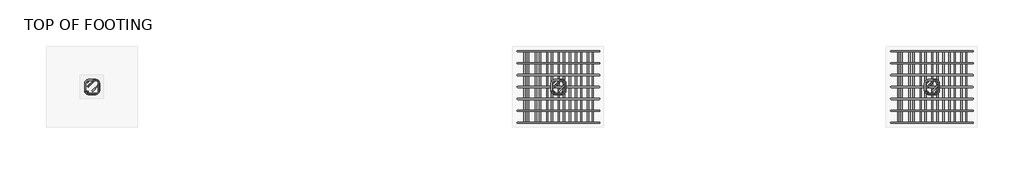
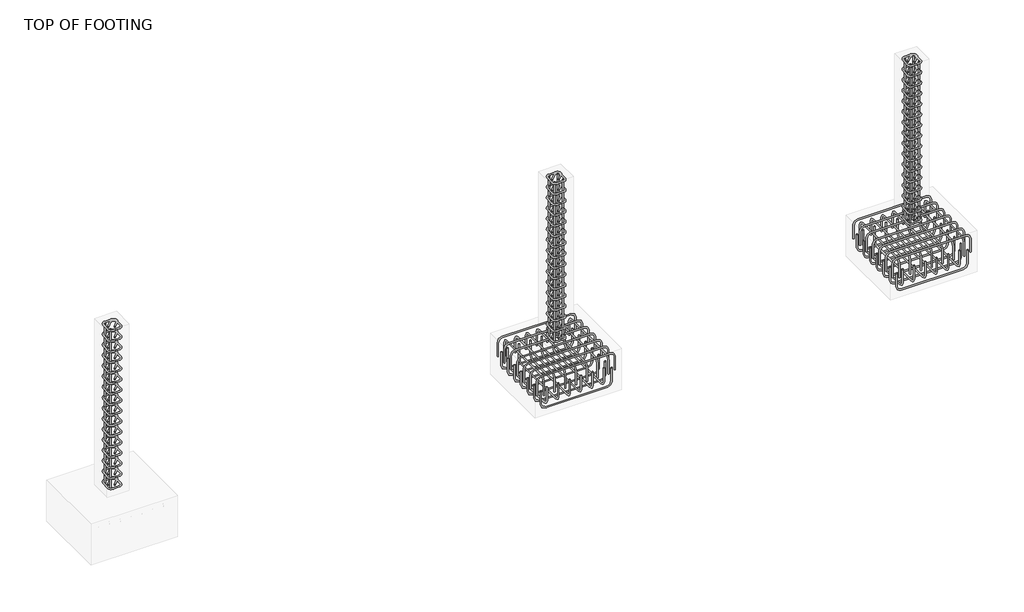
# One storey, part 6 of 6: 16 reinforcing bars.
"""IFC4 building model written with IfcOpenShell, lengths in millimetres."""

from ifc_helpers import new_model, si_unit, point, frame, origin, place, context, project, spatial, polyline, circle_curve, trimmed, segment, composite_curve, source, transform, mapped, element, save
from ifc_brep_helpers import swept_disk

model = new_model("IFC4")

# Units and contexts
model_context = context("Model", 3, world=origin())
ifc_project = project(units=[si_unit("LENGTHUNIT", "METRE", prefix="MILLI")], contexts=[model_context])

# Site, building, storey
site = spatial("IfcSite", under=ifc_project)
building = spatial("IfcBuilding", under=site)
storey = spatial("IfcBuildingStorey", under=building, Name="TOP OF FOOTING", Elevation=-1828.8)

# Reinforcing bars
placement = place(None, origin())
reinforcing_bar_shape = source(origin(), model_context, "Body", "SolidModel", [
    swept_disk(composite_curve([segment(polyline([(-6942.8971795, 4666.2516651, -2038.8), (-6942.8971795, 4666.2516651, -2186.1)]), True, "CONTINUOUS"), segment(trimmed(circle_curve(frame((-6989.2471795, 4666.2516651, -2186.1), z_axis=(0.0, 1.0, 0.0), x_axis=(46.350000000000364, 0.0, 0.0)), 46.35), [point((-6942.8971795, 4666.2516651, -2186.1))], [point((-6989.2471795, 4666.2516651, -2232.45))], True, "CARTESIAN"), True, "CONTINUOUS"), segment(polyline([(-6989.2471795, 4666.2516651, -2232.45), (-7632.3877906, 4666.2516651, -2232.45)]), True, "CONTINUOUS"), segment(trimmed(circle_curve(frame((-7632.3877906, 4666.2516651, -2186.1), z_axis=(0.0, 1.0, 0.0), x_axis=(0.0, 0.0, -46.34999999999991)), 46.35), [point((-7632.3877906, 4666.2516651, -2232.45))], [point((-7678.7377906, 4666.2516651, -2186.1))], True, "CARTESIAN"), True, "CONTINUOUS"), segment(polyline([(-7678.7377906, 4666.2516651, -2186.1), (-7678.7377906, 4666.2516651, -2038.8)]), True, "CONTINUOUS")], self_intersect=False), 6.35),
])
element("IfcReinforcingBar", 1, at=placement, inside=storey, context=model_context, shape_type="MappedRepresentation", body=[
    mapped(reinforcing_bar_shape, transform((0.0, 0.0, 0.0), x_axis=(1.0, 0.0, 0.0), y_axis=(0.0, 1.0, 0.0), z_axis=(0.0, 0.0, 1.0))),
    mapped(reinforcing_bar_shape, transform((0.0, -117.8833333, 0.0), x_axis=(1.0, 0.0, 0.0), y_axis=(0.0, 1.0, 0.0), z_axis=(0.0, 0.0, 1.0))),
    mapped(reinforcing_bar_shape, transform((0.0, -235.7666667, 0.0), x_axis=(1.0, 0.0, 0.0), y_axis=(0.0, 1.0, 0.0), z_axis=(0.0, 0.0, 1.0))),
    mapped(reinforcing_bar_shape, transform((0.0, -353.65, 0.0), x_axis=(1.0, 0.0, 0.0), y_axis=(0.0, 1.0, 0.0), z_axis=(0.0, 0.0, 1.0))),
    mapped(reinforcing_bar_shape, transform((0.0, -471.5333333, 0.0), x_axis=(1.0, 0.0, 0.0), y_axis=(0.0, 1.0, 0.0), z_axis=(0.0, 0.0, 1.0))),
    mapped(reinforcing_bar_shape, transform((0.0, -589.4166667, 0.0), x_axis=(1.0, 0.0, 0.0), y_axis=(0.0, 1.0, 0.0), z_axis=(0.0, 0.0, 1.0))),
    mapped(reinforcing_bar_shape, transform((0.0, -707.3, 0.0), x_axis=(1.0, 0.0, 0.0), y_axis=(0.0, 1.0, 0.0), z_axis=(0.0, 0.0, 1.0))),
])
reinforcing_bar_2_shape = source(origin(), model_context, "Body", "SolidModel", [
    swept_disk(composite_curve([segment(polyline([(-7718.1173382, 4666.2516651, -2070.9463075), (-7718.1173382, 4666.2516651, -1923.6463075)]), True, "CONTINUOUS"), segment(trimmed(circle_curve(frame((-7671.7673382, 4666.2516651, -1923.6463075), z_axis=(0.0, 1.0, 0.0), x_axis=(-46.349999999999454, 0.0, 0.0)), 46.35), [point((-7718.1173382, 4666.2516651, -1923.6463075))], [point((-7671.7673382, 4666.2516651, -1877.2963075))], True, "CARTESIAN"), True, "CONTINUOUS"), segment(polyline([(-7671.7673382, 4666.2516651, -1877.2963075), (-6957.1673382, 4666.2516651, -1877.2963075)]), True, "CONTINUOUS"), segment(trimmed(circle_curve(frame((-6957.1673382, 4666.2516651, -1923.6463075), z_axis=(0.0, 1.0, 0.0), x_axis=(0.0, 0.0, 46.34999999999991)), 46.35), [point((-6957.1673382, 4666.2516651, -1877.2963075))], [point((-6910.8173382, 4666.2516651, -1923.6463075))], True, "CARTESIAN"), True, "CONTINUOUS"), segment(polyline([(-6910.8173382, 4666.2516651, -1923.6463075), (-6910.8173382, 4666.2516651, -2070.9463075)]), True, "CONTINUOUS")], self_intersect=False), 6.35),
])
element("IfcReinforcingBar", 2, at=placement, inside=storey, context=model_context, shape_type="MappedRepresentation", body=[
    mapped(reinforcing_bar_2_shape, transform((0.0, 0.0, 0.0), x_axis=(1.0, 0.0, 0.0), y_axis=(0.0, 1.0, 0.0), z_axis=(0.0, 0.0, 1.0))),
    mapped(reinforcing_bar_2_shape, transform((0.0, -117.8833333, 0.0), x_axis=(1.0, 0.0, 0.0), y_axis=(0.0, 1.0, 0.0), z_axis=(0.0, 0.0, 1.0))),
    mapped(reinforcing_bar_2_shape, transform((0.0, -235.7666667, 0.0), x_axis=(1.0, 0.0, 0.0), y_axis=(0.0, 1.0, 0.0), z_axis=(0.0, 0.0, 1.0))),
    mapped(reinforcing_bar_2_shape, transform((0.0, -353.65, 0.0), x_axis=(1.0, 0.0, 0.0), y_axis=(0.0, 1.0, 0.0), z_axis=(0.0, 0.0, 1.0))),
    mapped(reinforcing_bar_2_shape, transform((0.0, -471.5333333, 0.0), x_axis=(1.0, 0.0, 0.0), y_axis=(0.0, 1.0, 0.0), z_axis=(0.0, 0.0, 1.0))),
    mapped(reinforcing_bar_2_shape, transform((0.0, -589.4166667, 0.0), x_axis=(1.0, 0.0, 0.0), y_axis=(0.0, 1.0, 0.0), z_axis=(0.0, 0.0, 1.0))),
    mapped(reinforcing_bar_2_shape, transform((0.0, -707.3, 0.0), x_axis=(1.0, 0.0, 0.0), y_axis=(0.0, 1.0, 0.0), z_axis=(0.0, 0.0, 1.0))),
])
reinforcing_bar_3_shape = source(origin(), model_context, "Body", "SolidModel", [
    swept_disk(composite_curve([segment(polyline([(-6975.9662545, 4666.2516651, -2094.0228735), (-6975.9662545, 4666.2516651, -1946.7228735)]), True, "CONTINUOUS"), segment(trimmed(circle_curve(frame((-6975.9662545, 4619.9016651, -1946.7228735), z_axis=(1.0, 0.0, 0.0), x_axis=(0.0, 46.349999999999454, 0.0)), 46.35), [point((-6975.9662545, 4666.2516651, -1946.7228735))], [point((-6975.9662545, 4619.9016651, -1900.3728735))], True, "CARTESIAN"), True, "CONTINUOUS"), segment(polyline([(-6975.9662545, 4619.9016651, -1900.3728735), (-6975.9662545, 4005.3016651, -1900.3728735)]), True, "CONTINUOUS"), segment(trimmed(circle_curve(frame((-6975.9662545, 4005.3016651, -1946.7228735), z_axis=(1.0, 0.0, 0.0), x_axis=(0.0, 0.0, 46.350000000000136)), 46.35), [point((-6975.9662545, 4005.3016651, -1900.3728735))], [point((-6975.9662545, 3958.9516651, -1946.7228735))], True, "CARTESIAN"), True, "CONTINUOUS"), segment(polyline([(-6975.9662545, 3958.9516651, -1946.7228735), (-6975.9662545, 3958.9516651, -2094.0228735)]), True, "CONTINUOUS")], self_intersect=False), 6.35),
])
element("IfcReinforcingBar", 3, at=placement, inside=storey, context=model_context, shape_type="MappedRepresentation", body=[
    mapped(reinforcing_bar_3_shape, transform((0.0, 0.0, 0.0), x_axis=(1.0, 0.0, 0.0), y_axis=(0.0, 1.0, 0.0), z_axis=(0.0, 0.0, 1.0))),
    mapped(reinforcing_bar_3_shape, transform((-112.124631, 0.0, 0.0), x_axis=(1.0, 0.0, 0.0), y_axis=(0.0, 1.0, 0.0), z_axis=(0.0, 0.0, 1.0))),
    mapped(reinforcing_bar_3_shape, transform((-224.2492621, 0.0, 0.0), x_axis=(1.0, 0.0, 0.0), y_axis=(0.0, 1.0, 0.0), z_axis=(0.0, 0.0, 1.0))),
    mapped(reinforcing_bar_3_shape, transform((-336.3738931, 0.0, 0.0), x_axis=(1.0, 0.0, 0.0), y_axis=(0.0, 1.0, 0.0), z_axis=(0.0, 0.0, 1.0))),
    mapped(reinforcing_bar_3_shape, transform((-448.4985241, 0.0, 0.0), x_axis=(1.0, 0.0, 0.0), y_axis=(0.0, 1.0, 0.0), z_axis=(0.0, 0.0, 1.0))),
    mapped(reinforcing_bar_3_shape, transform((-560.6231552, 0.0, 0.0), x_axis=(1.0, 0.0, 0.0), y_axis=(0.0, 1.0, 0.0), z_axis=(0.0, 0.0, 1.0))),
    mapped(reinforcing_bar_3_shape, transform((-672.7477862, 0.0, 0.0), x_axis=(1.0, 0.0, 0.0), y_axis=(0.0, 1.0, 0.0), z_axis=(0.0, 0.0, 1.0))),
])
reinforcing_bar_4_shape = source(origin(), model_context, "Body", "SolidModel", [
    swept_disk(composite_curve([segment(polyline([(-7615.9564967, 4666.2516651, -2014.7438142), (-7615.9564967, 4666.2516651, -2162.0438142)]), True, "CONTINUOUS"), segment(trimmed(circle_curve(frame((-7615.9564967, 4619.9016651, -2162.0438142), z_axis=(-1.0, 0.0, 0.0), x_axis=(0.0, 46.349999999999454, 0.0)), 46.35), [point((-7615.9564967, 4666.2516651, -2162.0438142))], [point((-7615.9564967, 4619.9016651, -2208.3938142))], True, "CARTESIAN"), True, "CONTINUOUS"), segment(polyline([(-7615.9564967, 4619.9016651, -2208.3938142), (-7615.9564967, 4005.3016651, -2208.3938142)]), True, "CONTINUOUS"), segment(trimmed(circle_curve(frame((-7615.9564967, 4005.3016651, -2162.0438142), z_axis=(-1.0, 0.0, 0.0), x_axis=(0.0, 0.0, -46.350000000000364)), 46.35), [point((-7615.9564967, 4005.3016651, -2208.3938142))], [point((-7615.9564967, 3958.9516651, -2162.0438142))], True, "CARTESIAN"), True, "CONTINUOUS"), segment(polyline([(-7615.9564967, 3958.9516651, -2162.0438142), (-7615.9564967, 3958.9516651, -2014.7438142)]), True, "CONTINUOUS")], self_intersect=False), 6.35),
])
element("IfcReinforcingBar", 4, at=placement, inside=storey, context=model_context, shape_type="MappedRepresentation", body=[
    mapped(reinforcing_bar_4_shape, transform((0.0, 0.0, 0.0), x_axis=(1.0, 0.0, 0.0), y_axis=(0.0, 1.0, 0.0), z_axis=(0.0, 0.0, 1.0))),
    mapped(reinforcing_bar_4_shape, transform((118.647936, 0.0, 0.0), x_axis=(1.0, 0.0, 0.0), y_axis=(0.0, 1.0, 0.0), z_axis=(0.0, 0.0, 1.0))),
    mapped(reinforcing_bar_4_shape, transform((237.295872, 0.0, 0.0), x_axis=(1.0, 0.0, 0.0), y_axis=(0.0, 1.0, 0.0), z_axis=(0.0, 0.0, 1.0))),
    mapped(reinforcing_bar_4_shape, transform((355.943808, 0.0, 0.0), x_axis=(1.0, 0.0, 0.0), y_axis=(0.0, 1.0, 0.0), z_axis=(0.0, 0.0, 1.0))),
    mapped(reinforcing_bar_4_shape, transform((474.591744, 0.0, 0.0), x_axis=(1.0, 0.0, 0.0), y_axis=(0.0, 1.0, 0.0), z_axis=(0.0, 0.0, 1.0))),
    mapped(reinforcing_bar_4_shape, transform((593.23968, 0.0, 0.0), x_axis=(1.0, 0.0, 0.0), y_axis=(0.0, 1.0, 0.0), z_axis=(0.0, 0.0, 1.0))),
])
reinforcing_bar_5_shape = source(origin(), model_context, "Body", "SolidModel", [
    swept_disk(composite_curve([segment(polyline([(-3249.1855212, 4666.2516651, -2038.8), (-3249.1855212, 4666.2516651, -2186.1)]), True, "CONTINUOUS"), segment(trimmed(circle_curve(frame((-3295.5355212, 4666.2516651, -2186.1), z_axis=(0.0, 1.0, 0.0), x_axis=(46.34999999999991, 0.0, 0.0)), 46.35), [point((-3249.1855212, 4666.2516651, -2186.1))], [point((-3295.5355212, 4666.2516651, -2232.45))], True, "CARTESIAN"), True, "CONTINUOUS"), segment(polyline([(-3295.5355212, 4666.2516651, -2232.45), (-3938.6761323, 4666.2516651, -2232.45)]), True, "CONTINUOUS"), segment(trimmed(circle_curve(frame((-3938.6761323, 4666.2516651, -2186.1), z_axis=(0.0, 1.0, 0.0), x_axis=(0.0, 0.0, -46.34999999999991)), 46.35), [point((-3938.6761323, 4666.2516651, -2232.45))], [point((-3985.0261323, 4666.2516651, -2186.1))], True, "CARTESIAN"), True, "CONTINUOUS"), segment(polyline([(-3985.0261323, 4666.2516651, -2186.1), (-3985.0261323, 4666.2516651, -2038.8)]), True, "CONTINUOUS")], self_intersect=False), 6.35),
])
element("IfcReinforcingBar", 5, at=placement, inside=storey, context=model_context, shape_type="MappedRepresentation", body=[
    mapped(reinforcing_bar_5_shape, transform((0.0, 0.0, 0.0), x_axis=(1.0, 0.0, 0.0), y_axis=(0.0, 1.0, 0.0), z_axis=(0.0, 0.0, 1.0))),
    mapped(reinforcing_bar_5_shape, transform((0.0, -117.8833333, 0.0), x_axis=(1.0, 0.0, 0.0), y_axis=(0.0, 1.0, 0.0), z_axis=(0.0, 0.0, 1.0))),
    mapped(reinforcing_bar_5_shape, transform((0.0, -235.7666667, 0.0), x_axis=(1.0, 0.0, 0.0), y_axis=(0.0, 1.0, 0.0), z_axis=(0.0, 0.0, 1.0))),
    mapped(reinforcing_bar_5_shape, transform((0.0, -353.65, 0.0), x_axis=(1.0, 0.0, 0.0), y_axis=(0.0, 1.0, 0.0), z_axis=(0.0, 0.0, 1.0))),
    mapped(reinforcing_bar_5_shape, transform((0.0, -471.5333333, 0.0), x_axis=(1.0, 0.0, 0.0), y_axis=(0.0, 1.0, 0.0), z_axis=(0.0, 0.0, 1.0))),
    mapped(reinforcing_bar_5_shape, transform((0.0, -589.4166667, 0.0), x_axis=(1.0, 0.0, 0.0), y_axis=(0.0, 1.0, 0.0), z_axis=(0.0, 0.0, 1.0))),
    mapped(reinforcing_bar_5_shape, transform((0.0, -707.3, 0.0), x_axis=(1.0, 0.0, 0.0), y_axis=(0.0, 1.0, 0.0), z_axis=(0.0, 0.0, 1.0))),
])
reinforcing_bar_6_shape = source(origin(), model_context, "Body", "SolidModel", [
    swept_disk(composite_curve([segment(polyline([(-4024.4056799, 4666.2516651, -2070.9463075), (-4024.4056799, 4666.2516651, -1923.6463075)]), True, "CONTINUOUS"), segment(trimmed(circle_curve(frame((-3978.0556799, 4666.2516651, -1923.6463075), z_axis=(0.0, 1.0, 0.0), x_axis=(-46.34999999999991, 0.0, 0.0)), 46.35), [point((-4024.4056799, 4666.2516651, -1923.6463075))], [point((-3978.0556799, 4666.2516651, -1877.2963075))], True, "CARTESIAN"), True, "CONTINUOUS"), segment(polyline([(-3978.0556799, 4666.2516651, -1877.2963075), (-3263.4556799, 4666.2516651, -1877.2963075)]), True, "CONTINUOUS"), segment(trimmed(circle_curve(frame((-3263.4556799, 4666.2516651, -1923.6463075), z_axis=(0.0, 1.0, 0.0), x_axis=(0.0, 0.0, 46.34999999999991)), 46.35), [point((-3263.4556799, 4666.2516651, -1877.2963075))], [point((-3217.1056799, 4666.2516651, -1923.6463075))], True, "CARTESIAN"), True, "CONTINUOUS"), segment(polyline([(-3217.1056799, 4666.2516651, -1923.6463075), (-3217.1056799, 4666.2516651, -2070.9463075)]), True, "CONTINUOUS")], self_intersect=False), 6.35),
])
element("IfcReinforcingBar", 6, at=placement, inside=storey, context=model_context, shape_type="MappedRepresentation", body=[
    mapped(reinforcing_bar_6_shape, transform((0.0, 0.0, 0.0), x_axis=(1.0, 0.0, 0.0), y_axis=(0.0, 1.0, 0.0), z_axis=(0.0, 0.0, 1.0))),
    mapped(reinforcing_bar_6_shape, transform((0.0, -117.8833333, 0.0), x_axis=(1.0, 0.0, 0.0), y_axis=(0.0, 1.0, 0.0), z_axis=(0.0, 0.0, 1.0))),
    mapped(reinforcing_bar_6_shape, transform((0.0, -235.7666667, 0.0), x_axis=(1.0, 0.0, 0.0), y_axis=(0.0, 1.0, 0.0), z_axis=(0.0, 0.0, 1.0))),
    mapped(reinforcing_bar_6_shape, transform((0.0, -353.65, 0.0), x_axis=(1.0, 0.0, 0.0), y_axis=(0.0, 1.0, 0.0), z_axis=(0.0, 0.0, 1.0))),
    mapped(reinforcing_bar_6_shape, transform((0.0, -471.5333333, 0.0), x_axis=(1.0, 0.0, 0.0), y_axis=(0.0, 1.0, 0.0), z_axis=(0.0, 0.0, 1.0))),
    mapped(reinforcing_bar_6_shape, transform((0.0, -589.4166667, 0.0), x_axis=(1.0, 0.0, 0.0), y_axis=(0.0, 1.0, 0.0), z_axis=(0.0, 0.0, 1.0))),
    mapped(reinforcing_bar_6_shape, transform((0.0, -707.3, 0.0), x_axis=(1.0, 0.0, 0.0), y_axis=(0.0, 1.0, 0.0), z_axis=(0.0, 0.0, 1.0))),
])
reinforcing_bar_7_shape = source(origin(), model_context, "Body", "SolidModel", [
    swept_disk(composite_curve([segment(polyline([(-3282.2545962, 4666.2516651, -2094.0228735), (-3282.2545962, 4666.2516651, -1946.7228735)]), True, "CONTINUOUS"), segment(trimmed(circle_curve(frame((-3282.2545962, 4619.9016651, -1946.7228735), z_axis=(1.0, 0.0, 0.0), x_axis=(0.0, 46.349999999999454, 0.0)), 46.35), [point((-3282.2545962, 4666.2516651, -1946.7228735))], [point((-3282.2545962, 4619.9016651, -1900.3728735))], True, "CARTESIAN"), True, "CONTINUOUS"), segment(polyline([(-3282.2545962, 4619.9016651, -1900.3728735), (-3282.2545962, 4005.3016651, -1900.3728735)]), True, "CONTINUOUS"), segment(trimmed(circle_curve(frame((-3282.2545962, 4005.3016651, -1946.7228735), z_axis=(1.0, 0.0, 0.0), x_axis=(0.0, 0.0, 46.350000000000136)), 46.35), [point((-3282.2545962, 4005.3016651, -1900.3728735))], [point((-3282.2545962, 3958.9516651, -1946.7228735))], True, "CARTESIAN"), True, "CONTINUOUS"), segment(polyline([(-3282.2545962, 3958.9516651, -1946.7228735), (-3282.2545962, 3958.9516651, -2094.0228735)]), True, "CONTINUOUS")], self_intersect=False), 6.35),
])
element("IfcReinforcingBar", 7, at=placement, inside=storey, context=model_context, shape_type="MappedRepresentation", body=[
    mapped(reinforcing_bar_7_shape, transform((0.0, 0.0, 0.0), x_axis=(1.0, 0.0, 0.0), y_axis=(0.0, 1.0, 0.0), z_axis=(0.0, 0.0, 1.0))),
    mapped(reinforcing_bar_7_shape, transform((-112.124631, 0.0, 0.0), x_axis=(1.0, 0.0, 0.0), y_axis=(0.0, 1.0, 0.0), z_axis=(0.0, 0.0, 1.0))),
    mapped(reinforcing_bar_7_shape, transform((-224.2492621, 0.0, 0.0), x_axis=(1.0, 0.0, 0.0), y_axis=(0.0, 1.0, 0.0), z_axis=(0.0, 0.0, 1.0))),
    mapped(reinforcing_bar_7_shape, transform((-336.3738931, 0.0, 0.0), x_axis=(1.0, 0.0, 0.0), y_axis=(0.0, 1.0, 0.0), z_axis=(0.0, 0.0, 1.0))),
    mapped(reinforcing_bar_7_shape, transform((-448.4985241, 0.0, 0.0), x_axis=(1.0, 0.0, 0.0), y_axis=(0.0, 1.0, 0.0), z_axis=(0.0, 0.0, 1.0))),
    mapped(reinforcing_bar_7_shape, transform((-560.6231552, 0.0, 0.0), x_axis=(1.0, 0.0, 0.0), y_axis=(0.0, 1.0, 0.0), z_axis=(0.0, 0.0, 1.0))),
    mapped(reinforcing_bar_7_shape, transform((-672.7477862, 0.0, 0.0), x_axis=(1.0, 0.0, 0.0), y_axis=(0.0, 1.0, 0.0), z_axis=(0.0, 0.0, 1.0))),
])
reinforcing_bar_8_shape = source(origin(), model_context, "Body", "SolidModel", [
    swept_disk(composite_curve([segment(polyline([(-3922.2448384, 4666.2516651, -2014.7438142), (-3922.2448384, 4666.2516651, -2162.0438142)]), True, "CONTINUOUS"), segment(trimmed(circle_curve(frame((-3922.2448384, 4619.9016651, -2162.0438142), z_axis=(-1.0, 0.0, 0.0), x_axis=(0.0, 46.349999999999454, 0.0)), 46.35), [point((-3922.2448384, 4666.2516651, -2162.0438142))], [point((-3922.2448384, 4619.9016651, -2208.3938142))], True, "CARTESIAN"), True, "CONTINUOUS"), segment(polyline([(-3922.2448384, 4619.9016651, -2208.3938142), (-3922.2448384, 4005.3016651, -2208.3938142)]), True, "CONTINUOUS"), segment(trimmed(circle_curve(frame((-3922.2448384, 4005.3016651, -2162.0438142), z_axis=(-1.0, 0.0, 0.0), x_axis=(0.0, 0.0, -46.350000000000364)), 46.35), [point((-3922.2448384, 4005.3016651, -2208.3938142))], [point((-3922.2448384, 3958.9516651, -2162.0438142))], True, "CARTESIAN"), True, "CONTINUOUS"), segment(polyline([(-3922.2448384, 3958.9516651, -2162.0438142), (-3922.2448384, 3958.9516651, -2014.7438142)]), True, "CONTINUOUS")], self_intersect=False), 6.35),
])
element("IfcReinforcingBar", 8, at=placement, inside=storey, context=model_context, shape_type="MappedRepresentation", body=[
    mapped(reinforcing_bar_8_shape, transform((0.0, 0.0, 0.0), x_axis=(1.0, 0.0, 0.0), y_axis=(0.0, 1.0, 0.0), z_axis=(0.0, 0.0, 1.0))),
    mapped(reinforcing_bar_8_shape, transform((118.647936, 0.0, 0.0), x_axis=(1.0, 0.0, 0.0), y_axis=(0.0, 1.0, 0.0), z_axis=(0.0, 0.0, 1.0))),
    mapped(reinforcing_bar_8_shape, transform((237.295872, 0.0, 0.0), x_axis=(1.0, 0.0, 0.0), y_axis=(0.0, 1.0, 0.0), z_axis=(0.0, 0.0, 1.0))),
    mapped(reinforcing_bar_8_shape, transform((355.943808, 0.0, 0.0), x_axis=(1.0, 0.0, 0.0), y_axis=(0.0, 1.0, 0.0), z_axis=(0.0, 0.0, 1.0))),
    mapped(reinforcing_bar_8_shape, transform((474.591744, 0.0, 0.0), x_axis=(1.0, 0.0, 0.0), y_axis=(0.0, 1.0, 0.0), z_axis=(0.0, 0.0, 1.0))),
    mapped(reinforcing_bar_8_shape, transform((593.23968, 0.0, 0.0), x_axis=(1.0, 0.0, 0.0), y_axis=(0.0, 1.0, 0.0), z_axis=(0.0, 0.0, 1.0))),
])
reinforcing_bar_9_shape = source(origin(), model_context, "Body", "SolidModel", [
    swept_disk(composite_curve([segment(polyline([(-3576.0006936, 4361.3993608, -40.0), (-3576.0006936, 4361.3993608, -1788.8)]), True, "CONTINUOUS")], self_intersect=False), 6.35),
])
element("IfcReinforcingBar", 9, at=placement, inside=storey, context=model_context, shape_type="MappedRepresentation", body=[
    mapped(reinforcing_bar_9_shape, transform((0.0, 0.0, 0.0), x_axis=(1.0, 0.0, 0.0), y_axis=(0.0, 1.0, 0.0), z_axis=(0.0, 0.0, 1.0))),
    mapped(reinforcing_bar_9_shape, transform((0.0, -96.9916148, 0.0), x_axis=(1.0, 0.0, 0.0), y_axis=(0.0, 1.0, 0.0), z_axis=(0.0, 0.0, 1.0))),
])
reinforcing_bar_10_shape = source(origin(), model_context, "Body", "SolidModel", [
    swept_disk(composite_curve([segment(polyline([(-3662.0670404, 4315.6258997, -46.35), (-3606.3234775, 4371.3694627, -46.35)]), True, "CONTINUOUS"), segment(trimmed(circle_curve(frame((-3584.1556799, 4349.2016651, -46.35), z_axis=(0.0, 0.0, -1.0), x_axis=(-22.167797600000085, 22.167797600000085, 0.0)), 31.35), [point((-3606.3234775, 4371.3694627, -46.35))], [point((-3552.8056799, 4349.2016651, -46.35))], True, "CARTESIAN"), True, "CONTINUOUS"), segment(polyline([(-3552.8056799, 4349.2016651, -46.35), (-3552.8056799, 4276.0016651, -46.35)]), True, "CONTINUOUS"), segment(trimmed(circle_curve(frame((-3584.1556799, 4276.0016651, -46.35), z_axis=(0.0, 0.0, -1.0), x_axis=(31.34999999999991, 0.0, 0.0)), 31.35), [point((-3552.8056799, 4276.0016651, -46.35))], [point((-3584.1556799, 4244.6516651, -46.35))], True, "CARTESIAN"), True, "CONTINUOUS"), segment(polyline([(-3584.1556799, 4244.6516651, -46.35), (-3657.3556799, 4244.6516651, -46.35)]), True, "CONTINUOUS"), segment(trimmed(circle_curve(frame((-3657.3556799, 4275.8656639, -43.4330185), z_axis=(0.0, 0.09304566152621355, -0.9956618426308951), x_axis=(0.0, -31.2139987999999, -2.9169814999999986)), 31.35), [point((-3657.3556799, 4244.6516651, -46.35))], [point((-3688.7056799, 4275.8656639, -43.4330185))], True, "CARTESIAN"), True, "CONTINUOUS"), segment(polyline([(-3688.7056799, 4275.8656639, -43.4330185), (-3688.7056799, 4349.3376663, -36.5669815)]), True, "CONTINUOUS"), segment(trimmed(circle_curve(frame((-3657.3556799, 4349.3376663, -36.5669815), z_axis=(0.0, 0.09304566152621355, -0.9956618426308951), x_axis=(-31.350000000000364, 0.0, 0.0)), 31.35), [point((-3688.7056799, 4349.3376663, -36.5669815))], [point((-3657.3556799, 4380.5516651, -33.65))], True, "CARTESIAN"), True, "CONTINUOUS"), segment(polyline([(-3657.3556799, 4380.5516651, -33.65), (-3584.1556799, 4380.5516651, -33.65)]), True, "CONTINUOUS"), segment(trimmed(circle_curve(frame((-3584.1556799, 4349.2016651, -33.65), z_axis=(0.0, 0.0, -1.0), x_axis=(0.0, 31.349999999999454, 0.0)), 31.35), [point((-3584.1556799, 4380.5516651, -33.65))], [point((-3561.9878823, 4327.0338675, -33.65))], True, "CARTESIAN"), True, "CONTINUOUS"), segment(polyline([(-3561.9878823, 4327.0338675, -33.65), (-3617.7314452, 4271.2903046, -33.65)]), True, "CONTINUOUS")], self_intersect=False), 6.35),
])
element("IfcReinforcingBar", 10, at=placement, inside=storey, context=model_context, shape_type="MappedRepresentation", body=[
    mapped(reinforcing_bar_10_shape, transform((0.0, 0.0, 0.0), x_axis=(1.0, 0.0, 0.0), y_axis=(0.0, 1.0, 0.0), z_axis=(0.0, 0.0, 1.0))),
    mapped(reinforcing_bar_10_shape, transform((0.0, 0.0, -115.74), x_axis=(1.0, 0.0, 0.0), y_axis=(0.0, 1.0, 0.0), z_axis=(0.0, 0.0, 1.0))),
    mapped(reinforcing_bar_10_shape, transform((0.0, 0.0, -231.48), x_axis=(1.0, 0.0, 0.0), y_axis=(0.0, 1.0, 0.0), z_axis=(0.0, 0.0, 1.0))),
    mapped(reinforcing_bar_10_shape, transform((0.0, 0.0, -347.22), x_axis=(1.0, 0.0, 0.0), y_axis=(0.0, 1.0, 0.0), z_axis=(0.0, 0.0, 1.0))),
    mapped(reinforcing_bar_10_shape, transform((0.0, 0.0, -462.96), x_axis=(1.0, 0.0, 0.0), y_axis=(0.0, 1.0, 0.0), z_axis=(0.0, 0.0, 1.0))),
    mapped(reinforcing_bar_10_shape, transform((0.0, 0.0, -578.7), x_axis=(1.0, 0.0, 0.0), y_axis=(0.0, 1.0, 0.0), z_axis=(0.0, 0.0, 1.0))),
    mapped(reinforcing_bar_10_shape, transform((0.0, 0.0, -694.44), x_axis=(1.0, 0.0, 0.0), y_axis=(0.0, 1.0, 0.0), z_axis=(0.0, 0.0, 1.0))),
    mapped(reinforcing_bar_10_shape, transform((0.0, 0.0, -810.18), x_axis=(1.0, 0.0, 0.0), y_axis=(0.0, 1.0, 0.0), z_axis=(0.0, 0.0, 1.0))),
    mapped(reinforcing_bar_10_shape, transform((0.0, 0.0, -925.92), x_axis=(1.0, 0.0, 0.0), y_axis=(0.0, 1.0, 0.0), z_axis=(0.0, 0.0, 1.0))),
    mapped(reinforcing_bar_10_shape, transform((0.0, 0.0, -1041.66), x_axis=(1.0, 0.0, 0.0), y_axis=(0.0, 1.0, 0.0), z_axis=(0.0, 0.0, 1.0))),
    mapped(reinforcing_bar_10_shape, transform((0.0, 0.0, -1157.4), x_axis=(1.0, 0.0, 0.0), y_axis=(0.0, 1.0, 0.0), z_axis=(0.0, 0.0, 1.0))),
    mapped(reinforcing_bar_10_shape, transform((0.0, 0.0, -1273.14), x_axis=(1.0, 0.0, 0.0), y_axis=(0.0, 1.0, 0.0), z_axis=(0.0, 0.0, 1.0))),
    mapped(reinforcing_bar_10_shape, transform((0.0, 0.0, -1388.88), x_axis=(1.0, 0.0, 0.0), y_axis=(0.0, 1.0, 0.0), z_axis=(0.0, 0.0, 1.0))),
    mapped(reinforcing_bar_10_shape, transform((0.0, 0.0, -1504.62), x_axis=(1.0, 0.0, 0.0), y_axis=(0.0, 1.0, 0.0), z_axis=(0.0, 0.0, 1.0))),
    mapped(reinforcing_bar_10_shape, transform((0.0, 0.0, -1620.36), x_axis=(1.0, 0.0, 0.0), y_axis=(0.0, 1.0, 0.0), z_axis=(0.0, 0.0, 1.0))),
    mapped(reinforcing_bar_10_shape, transform((0.0, 0.0, -1736.1), x_axis=(1.0, 0.0, 0.0), y_axis=(0.0, 1.0, 0.0), z_axis=(0.0, 0.0, 1.0))),
])
reinforcing_bar_11_shape = source(origin(), model_context, "Body", "SolidModel", [
    swept_disk(composite_curve([segment(polyline([(-3665.5106662, 4361.3993608, -40.0), (-3665.5106662, 4361.3993608, -1788.8)]), True, "CONTINUOUS")], self_intersect=False), 6.35),
])
element("IfcReinforcingBar", 11, at=placement, inside=storey, context=model_context, shape_type="MappedRepresentation", body=[
    mapped(reinforcing_bar_11_shape, transform((0.0, 0.0, 0.0), x_axis=(1.0, 0.0, 0.0), y_axis=(0.0, 1.0, 0.0), z_axis=(0.0, 0.0, 1.0))),
    mapped(reinforcing_bar_11_shape, transform((0.0, -96.9916148, 0.0), x_axis=(1.0, 0.0, 0.0), y_axis=(0.0, 1.0, 0.0), z_axis=(0.0, 0.0, 1.0))),
])
reinforcing_bar_12_shape = source(origin(), model_context, "Body", "SolidModel", [
    swept_disk(composite_curve([segment(polyline([(-7269.7123519, 4361.3993608, -40.0), (-7269.7123519, 4361.3993608, -1788.8)]), True, "CONTINUOUS")], self_intersect=False), 6.35),
])
element("IfcReinforcingBar", 12, at=placement, inside=storey, context=model_context, shape_type="MappedRepresentation", body=[
    mapped(reinforcing_bar_12_shape, transform((0.0, 0.0, 0.0), x_axis=(1.0, 0.0, 0.0), y_axis=(0.0, 1.0, 0.0), z_axis=(0.0, 0.0, 1.0))),
    mapped(reinforcing_bar_12_shape, transform((0.0, -96.9916148, 0.0), x_axis=(1.0, 0.0, 0.0), y_axis=(0.0, 1.0, 0.0), z_axis=(0.0, 0.0, 1.0))),
])
reinforcing_bar_13_shape = source(origin(), model_context, "Body", "SolidModel", [
    swept_disk(composite_curve([segment(polyline([(-7355.7786987, 4315.6258997, -46.35), (-7300.0351358, 4371.3694627, -46.35)]), True, "CONTINUOUS"), segment(trimmed(circle_curve(frame((-7277.8673382, 4349.2016651, -46.35), z_axis=(0.0, 0.0, -1.0), x_axis=(-22.167797600000085, 22.167797600000085, 0.0)), 31.35), [point((-7300.0351358, 4371.3694627, -46.35))], [point((-7246.5173382, 4349.2016651, -46.35))], True, "CARTESIAN"), True, "CONTINUOUS"), segment(polyline([(-7246.5173382, 4349.2016651, -46.35), (-7246.5173382, 4276.0016651, -46.35)]), True, "CONTINUOUS"), segment(trimmed(circle_curve(frame((-7277.8673382, 4276.0016651, -46.35), z_axis=(0.0, 0.0, -1.0), x_axis=(31.349999999999454, 0.0, 0.0)), 31.35), [point((-7246.5173382, 4276.0016651, -46.35))], [point((-7277.8673382, 4244.6516651, -46.35))], True, "CARTESIAN"), True, "CONTINUOUS"), segment(polyline([(-7277.8673382, 4244.6516651, -46.35), (-7351.0673382, 4244.6516651, -46.35)]), True, "CONTINUOUS"), segment(trimmed(circle_curve(frame((-7351.0673382, 4275.8656639, -43.4330185), z_axis=(0.0, 0.09304566152621355, -0.9956618426308951), x_axis=(0.0, -31.2139987999999, -2.9169814999999986)), 31.35), [point((-7351.0673382, 4244.6516651, -46.35))], [point((-7382.4173382, 4275.8656639, -43.4330185))], True, "CARTESIAN"), True, "CONTINUOUS"), segment(polyline([(-7382.4173382, 4275.8656639, -43.4330185), (-7382.4173382, 4349.3376663, -36.5669815)]), True, "CONTINUOUS"), segment(trimmed(circle_curve(frame((-7351.0673382, 4349.3376663, -36.5669815), z_axis=(0.0, 0.09304566152621355, -0.9956618426308951), x_axis=(-31.349999999999454, 0.0, 0.0)), 31.35), [point((-7382.4173382, 4349.3376663, -36.5669815))], [point((-7351.0673382, 4380.5516651, -33.65))], True, "CARTESIAN"), True, "CONTINUOUS"), segment(polyline([(-7351.0673382, 4380.5516651, -33.65), (-7277.8673382, 4380.5516651, -33.65)]), True, "CONTINUOUS"), segment(trimmed(circle_curve(frame((-7277.8673382, 4349.2016651, -33.65), z_axis=(0.0, 0.0, -1.0), x_axis=(0.0, 31.349999999999454, 0.0)), 31.35), [point((-7277.8673382, 4380.5516651, -33.65))], [point((-7255.6995406, 4327.0338675, -33.65))], True, "CARTESIAN"), True, "CONTINUOUS"), segment(polyline([(-7255.6995406, 4327.0338675, -33.65), (-7311.4431035, 4271.2903046, -33.65)]), True, "CONTINUOUS")], self_intersect=False), 6.35),
])
element("IfcReinforcingBar", 13, at=placement, inside=storey, context=model_context, shape_type="MappedRepresentation", body=[
    mapped(reinforcing_bar_13_shape, transform((0.0, 0.0, 0.0), x_axis=(1.0, 0.0, 0.0), y_axis=(0.0, 1.0, 0.0), z_axis=(0.0, 0.0, 1.0))),
    mapped(reinforcing_bar_13_shape, transform((0.0, 0.0, -115.74), x_axis=(1.0, 0.0, 0.0), y_axis=(0.0, 1.0, 0.0), z_axis=(0.0, 0.0, 1.0))),
    mapped(reinforcing_bar_13_shape, transform((0.0, 0.0, -231.48), x_axis=(1.0, 0.0, 0.0), y_axis=(0.0, 1.0, 0.0), z_axis=(0.0, 0.0, 1.0))),
    mapped(reinforcing_bar_13_shape, transform((0.0, 0.0, -347.22), x_axis=(1.0, 0.0, 0.0), y_axis=(0.0, 1.0, 0.0), z_axis=(0.0, 0.0, 1.0))),
    mapped(reinforcing_bar_13_shape, transform((0.0, 0.0, -462.96), x_axis=(1.0, 0.0, 0.0), y_axis=(0.0, 1.0, 0.0), z_axis=(0.0, 0.0, 1.0))),
    mapped(reinforcing_bar_13_shape, transform((0.0, 0.0, -578.7), x_axis=(1.0, 0.0, 0.0), y_axis=(0.0, 1.0, 0.0), z_axis=(0.0, 0.0, 1.0))),
    mapped(reinforcing_bar_13_shape, transform((0.0, 0.0, -694.44), x_axis=(1.0, 0.0, 0.0), y_axis=(0.0, 1.0, 0.0), z_axis=(0.0, 0.0, 1.0))),
    mapped(reinforcing_bar_13_shape, transform((0.0, 0.0, -810.18), x_axis=(1.0, 0.0, 0.0), y_axis=(0.0, 1.0, 0.0), z_axis=(0.0, 0.0, 1.0))),
    mapped(reinforcing_bar_13_shape, transform((0.0, 0.0, -925.92), x_axis=(1.0, 0.0, 0.0), y_axis=(0.0, 1.0, 0.0), z_axis=(0.0, 0.0, 1.0))),
    mapped(reinforcing_bar_13_shape, transform((0.0, 0.0, -1041.66), x_axis=(1.0, 0.0, 0.0), y_axis=(0.0, 1.0, 0.0), z_axis=(0.0, 0.0, 1.0))),
    mapped(reinforcing_bar_13_shape, transform((0.0, 0.0, -1157.4), x_axis=(1.0, 0.0, 0.0), y_axis=(0.0, 1.0, 0.0), z_axis=(0.0, 0.0, 1.0))),
    mapped(reinforcing_bar_13_shape, transform((0.0, 0.0, -1273.14), x_axis=(1.0, 0.0, 0.0), y_axis=(0.0, 1.0, 0.0), z_axis=(0.0, 0.0, 1.0))),
    mapped(reinforcing_bar_13_shape, transform((0.0, 0.0, -1388.88), x_axis=(1.0, 0.0, 0.0), y_axis=(0.0, 1.0, 0.0), z_axis=(0.0, 0.0, 1.0))),
    mapped(reinforcing_bar_13_shape, transform((0.0, 0.0, -1504.62), x_axis=(1.0, 0.0, 0.0), y_axis=(0.0, 1.0, 0.0), z_axis=(0.0, 0.0, 1.0))),
    mapped(reinforcing_bar_13_shape, transform((0.0, 0.0, -1620.36), x_axis=(1.0, 0.0, 0.0), y_axis=(0.0, 1.0, 0.0), z_axis=(0.0, 0.0, 1.0))),
    mapped(reinforcing_bar_13_shape, transform((0.0, 0.0, -1736.1), x_axis=(1.0, 0.0, 0.0), y_axis=(0.0, 1.0, 0.0), z_axis=(0.0, 0.0, 1.0))),
])
reinforcing_bar_14_shape = source(origin(), model_context, "Body", "SolidModel", [
    swept_disk(composite_curve([segment(polyline([(-7359.2223245, 4361.3993608, -40.0), (-7359.2223245, 4361.3993608, -1788.8)]), True, "CONTINUOUS")], self_intersect=False), 6.35),
])
element("IfcReinforcingBar", 14, at=placement, inside=storey, context=model_context, shape_type="MappedRepresentation", body=[
    mapped(reinforcing_bar_14_shape, transform((0.0, 0.0, 0.0), x_axis=(1.0, 0.0, 0.0), y_axis=(0.0, 1.0, 0.0), z_axis=(0.0, 0.0, 1.0))),
    mapped(reinforcing_bar_14_shape, transform((0.0, -96.9916148, 0.0), x_axis=(1.0, 0.0, 0.0), y_axis=(0.0, 1.0, 0.0), z_axis=(0.0, 0.0, 1.0))),
])
reinforcing_bar_15_shape = source(origin(), model_context, "Body", "SolidModel", [
    swept_disk(composite_curve([segment(polyline([(-11967.8670404, 4315.6258997, -46.35), (-11912.1234775, 4371.3694627, -46.35)]), True, "CONTINUOUS"), segment(trimmed(circle_curve(frame((-11889.9556799, 4349.2016651, -46.35), z_axis=(0.0, 0.0, -1.0), x_axis=(-22.167797599999176, 22.167797600000085, 0.0)), 31.35), [point((-11912.1234775, 4371.3694627, -46.35))], [point((-11858.6056799, 4349.2016651, -46.35))], True, "CARTESIAN"), True, "CONTINUOUS"), segment(polyline([(-11858.6056799, 4349.2016651, -46.35), (-11858.6056799, 4276.0016651, -46.35)]), True, "CONTINUOUS"), segment(trimmed(circle_curve(frame((-11889.9556799, 4276.0016651, -46.35), z_axis=(0.0, 0.0, -1.0), x_axis=(31.350000000000364, 0.0, 0.0)), 31.35), [point((-11858.6056799, 4276.0016651, -46.35))], [point((-11889.9556799, 4244.6516651, -46.35))], True, "CARTESIAN"), True, "CONTINUOUS"), segment(polyline([(-11889.9556799, 4244.6516651, -46.35), (-11963.1556799, 4244.6516651, -46.35)]), True, "CONTINUOUS"), segment(trimmed(circle_curve(frame((-11963.1556799, 4275.8656639, -43.4330185), z_axis=(0.0, 0.09304566152621355, -0.9956618426308951), x_axis=(0.0, -31.2139987999999, -2.9169814999999986)), 31.35), [point((-11963.1556799, 4244.6516651, -46.35))], [point((-11994.5056799, 4275.8656639, -43.4330185))], True, "CARTESIAN"), True, "CONTINUOUS"), segment(polyline([(-11994.5056799, 4275.8656639, -43.4330185), (-11994.5056799, 4349.3376663, -36.5669815)]), True, "CONTINUOUS"), segment(trimmed(circle_curve(frame((-11963.1556799, 4349.3376663, -36.5669815), z_axis=(0.0, 0.09304566152621355, -0.9956618426308951), x_axis=(-31.349999999998545, 0.0, 0.0)), 31.35), [point((-11994.5056799, 4349.3376663, -36.5669815))], [point((-11963.1556799, 4380.5516651, -33.65))], True, "CARTESIAN"), True, "CONTINUOUS"), segment(polyline([(-11963.1556799, 4380.5516651, -33.65), (-11889.9556799, 4380.5516651, -33.65)]), True, "CONTINUOUS"), segment(trimmed(circle_curve(frame((-11889.9556799, 4349.2016651, -33.65), z_axis=(0.0, 0.0, -1.0), x_axis=(0.0, 31.349999999999454, 0.0)), 31.35), [point((-11889.9556799, 4380.5516651, -33.65))], [point((-11867.7878823, 4327.0338675, -33.65))], True, "CARTESIAN"), True, "CONTINUOUS"), segment(polyline([(-11867.7878823, 4327.0338675, -33.65), (-11923.5314452, 4271.2903046, -33.65)]), True, "CONTINUOUS")], self_intersect=False), 6.35),
])
element("IfcReinforcingBar", 15, at=placement, inside=storey, context=model_context, shape_type="MappedRepresentation", body=[
    mapped(reinforcing_bar_15_shape, transform((0.0, 0.0, 0.0), x_axis=(1.0, 0.0, 0.0), y_axis=(0.0, 1.0, 0.0), z_axis=(0.0, 0.0, 1.0))),
    mapped(reinforcing_bar_15_shape, transform((0.0, 0.0, -115.74), x_axis=(1.0, 0.0, 0.0), y_axis=(0.0, 1.0, 0.0), z_axis=(0.0, 0.0, 1.0))),
    mapped(reinforcing_bar_15_shape, transform((0.0, 0.0, -231.48), x_axis=(1.0, 0.0, 0.0), y_axis=(0.0, 1.0, 0.0), z_axis=(0.0, 0.0, 1.0))),
    mapped(reinforcing_bar_15_shape, transform((0.0, 0.0, -347.22), x_axis=(1.0, 0.0, 0.0), y_axis=(0.0, 1.0, 0.0), z_axis=(0.0, 0.0, 1.0))),
    mapped(reinforcing_bar_15_shape, transform((0.0, 0.0, -462.96), x_axis=(1.0, 0.0, 0.0), y_axis=(0.0, 1.0, 0.0), z_axis=(0.0, 0.0, 1.0))),
    mapped(reinforcing_bar_15_shape, transform((0.0, 0.0, -578.7), x_axis=(1.0, 0.0, 0.0), y_axis=(0.0, 1.0, 0.0), z_axis=(0.0, 0.0, 1.0))),
    mapped(reinforcing_bar_15_shape, transform((0.0, 0.0, -694.44), x_axis=(1.0, 0.0, 0.0), y_axis=(0.0, 1.0, 0.0), z_axis=(0.0, 0.0, 1.0))),
    mapped(reinforcing_bar_15_shape, transform((0.0, 0.0, -810.18), x_axis=(1.0, 0.0, 0.0), y_axis=(0.0, 1.0, 0.0), z_axis=(0.0, 0.0, 1.0))),
    mapped(reinforcing_bar_15_shape, transform((0.0, 0.0, -925.92), x_axis=(1.0, 0.0, 0.0), y_axis=(0.0, 1.0, 0.0), z_axis=(0.0, 0.0, 1.0))),
    mapped(reinforcing_bar_15_shape, transform((0.0, 0.0, -1041.66), x_axis=(1.0, 0.0, 0.0), y_axis=(0.0, 1.0, 0.0), z_axis=(0.0, 0.0, 1.0))),
    mapped(reinforcing_bar_15_shape, transform((0.0, 0.0, -1157.4), x_axis=(1.0, 0.0, 0.0), y_axis=(0.0, 1.0, 0.0), z_axis=(0.0, 0.0, 1.0))),
    mapped(reinforcing_bar_15_shape, transform((0.0, 0.0, -1273.14), x_axis=(1.0, 0.0, 0.0), y_axis=(0.0, 1.0, 0.0), z_axis=(0.0, 0.0, 1.0))),
    mapped(reinforcing_bar_15_shape, transform((0.0, 0.0, -1388.88), x_axis=(1.0, 0.0, 0.0), y_axis=(0.0, 1.0, 0.0), z_axis=(0.0, 0.0, 1.0))),
    mapped(reinforcing_bar_15_shape, transform((0.0, 0.0, -1504.62), x_axis=(1.0, 0.0, 0.0), y_axis=(0.0, 1.0, 0.0), z_axis=(0.0, 0.0, 1.0))),
    mapped(reinforcing_bar_15_shape, transform((0.0, 0.0, -1620.36), x_axis=(1.0, 0.0, 0.0), y_axis=(0.0, 1.0, 0.0), z_axis=(0.0, 0.0, 1.0))),
    mapped(reinforcing_bar_15_shape, transform((0.0, 0.0, -1736.1), x_axis=(1.0, 0.0, 0.0), y_axis=(0.0, 1.0, 0.0), z_axis=(0.0, 0.0, 1.0))),
])
reinforcing_bar_16_shape = source(origin(), model_context, "Body", "SolidModel", [
    swept_disk(composite_curve([segment(polyline([(-11971.3106662, 4361.3993608, -40.0), (-11971.3106662, 4361.3993608, -1788.8)]), True, "CONTINUOUS")], self_intersect=False), 6.35),
])
element("IfcReinforcingBar", 16, at=placement, inside=storey, context=model_context, shape_type="MappedRepresentation", body=[
    mapped(reinforcing_bar_16_shape, transform((0.0, 0.0, 0.0), x_axis=(1.0, 0.0, 0.0), y_axis=(0.0, 1.0, 0.0), z_axis=(0.0, 0.0, 1.0))),
    mapped(reinforcing_bar_16_shape, transform((0.0, -96.9916148, 0.0), x_axis=(1.0, 0.0, 0.0), y_axis=(0.0, 1.0, 0.0), z_axis=(0.0, 0.0, 1.0))),
])

save(model, "model.ifc")

# Revit data of these elements
# Elements 1, 2, 3, 4, 5, 6, 7, 8, 9, 10, 11, 12, 13, 14, 15, 16 (IfcReinforcingBar)
#   Phase Created = New Construction
